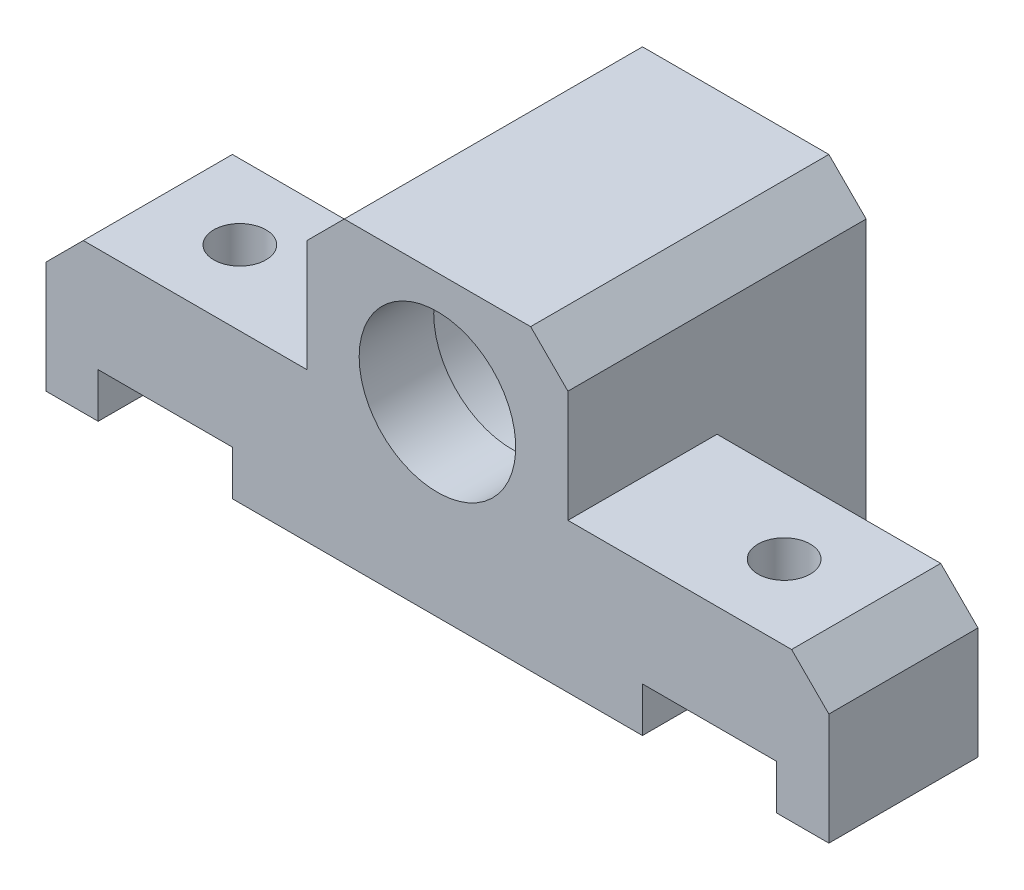
ISO-10303-21;
HEADER;
FILE_DESCRIPTION(('STEP AP214'),'2;1');
FILE_NAME('part.step','',(''),(''),'','','');
FILE_SCHEMA(('AUTOMOTIVE_DESIGN { 1 0 10303 214 1 1 1 1 }'));
ENDSEC;
DATA;
#1=APPLICATION_CONTEXT('core data for automotive mechanical design processes');
#2=APPLICATION_PROTOCOL_DEFINITION('international standard','automotive_design',2000,#1);
#3=PRODUCT_CONTEXT('',#1,'mechanical');
#4=PRODUCT('Part','Part','',(#3));
#5=PRODUCT_RELATED_PRODUCT_CATEGORY('part','',(#4));
#6=PRODUCT_DEFINITION_FORMATION('','',#4);
#7=PRODUCT_DEFINITION_CONTEXT('part definition',#1,'design');
#8=PRODUCT_DEFINITION('design','',#6,#7);
#9=PRODUCT_DEFINITION_SHAPE('','',#8);
#10=(LENGTH_UNIT() NAMED_UNIT(*) SI_UNIT(.MILLI.,.METRE.));
#11=(NAMED_UNIT(*) PLANE_ANGLE_UNIT() SI_UNIT($,.RADIAN.));
#12=(NAMED_UNIT(*) SI_UNIT($,.STERADIAN.) SOLID_ANGLE_UNIT());
#13=UNCERTAINTY_MEASURE_WITH_UNIT(LENGTH_MEASURE(1.E-05),#10,'distance_accuracy_value','');
#14=(GEOMETRIC_REPRESENTATION_CONTEXT(3) GLOBAL_UNCERTAINTY_ASSIGNED_CONTEXT((#13)) GLOBAL_UNIT_ASSIGNED_CONTEXT((#10,
#11,#12)) REPRESENTATION_CONTEXT('',''));
#15=CARTESIAN_POINT('',(0.,0.,0.));
#16=DIRECTION('',(0.,0.,1.));
#17=DIRECTION('',(1.,0.,0.));
#18=AXIS2_PLACEMENT_3D('',#15,#16,#17);
#19=CARTESIAN_POINT('',(0.,0.,40.));
#20=DIRECTION('',(0.,1.,0.));
#21=DIRECTION('',(0.,0.,1.));
#22=AXIS2_PLACEMENT_3D('',#19,#20,#21);
#23=PLANE('',#22);
#24=DIRECTION('',(1.,0.,0.));
#25=VECTOR('',#24,1.);
#26=CARTESIAN_POINT('',(-35.,0.,20.));
#27=LINE('',#26,#25);
#28=CARTESIAN_POINT('',(-35.,0.,20.));
#29=VERTEX_POINT('',#28);
#30=CARTESIAN_POINT('',(-28.,0.,20.));
#31=VERTEX_POINT('',#30);
#32=EDGE_CURVE('E286',#29,#31,#27,.T.);
#33=ORIENTED_EDGE('',*,*,#32,.T.);
#34=DIRECTION('',(0.,0.,-1.));
#35=VECTOR('',#34,1.);
#36=CARTESIAN_POINT('',(-28.,0.,40.));
#37=LINE('',#36,#35);
#38=CARTESIAN_POINT('',(-28.,0.,40.));
#39=VERTEX_POINT('',#38);
#40=EDGE_CURVE('E230',#39,#31,#37,.T.);
#41=ORIENTED_EDGE('',*,*,#40,.F.);
#42=DIRECTION('',(1.,0.,0.));
#43=VECTOR('',#42,1.);
#44=CARTESIAN_POINT('',(0.,0.,40.));
#45=LINE('',#44,#43);
#46=CARTESIAN_POINT('',(-35.,0.,40.));
#47=VERTEX_POINT('',#46);
#48=EDGE_CURVE('E327',#47,#39,#45,.T.);
#49=ORIENTED_EDGE('',*,*,#48,.F.);
#50=DIRECTION('',(0.,0.,1.));
#51=VECTOR('',#50,1.);
#52=CARTESIAN_POINT('',(-35.,0.,20.));
#53=LINE('',#52,#51);
#54=EDGE_CURVE('E313',#29,#47,#53,.T.);
#55=ORIENTED_EDGE('',*,*,#54,.F.);
#56=EDGE_LOOP('',(#33,#41,#49,#55));
#57=FACE_BOUND('',#56,.T.);
#58=ADVANCED_FACE('F44',(#57),#23,.F.);
#59=CARTESIAN_POINT('',(63.,0.,40.));
#60=VERTEX_POINT('',#59);
#61=CARTESIAN_POINT('',(70.,0.,40.));
#62=VERTEX_POINT('',#61);
#63=EDGE_CURVE('E330',#60,#62,#45,.T.);
#64=ORIENTED_EDGE('',*,*,#63,.F.);
#65=DIRECTION('',(0.,0.,-1.));
#66=VECTOR('',#65,1.);
#67=CARTESIAN_POINT('',(63.,0.,40.));
#68=LINE('',#67,#66);
#69=CARTESIAN_POINT('',(63.,0.,20.));
#70=VERTEX_POINT('',#69);
#71=EDGE_CURVE('E250',#60,#70,#68,.T.);
#72=ORIENTED_EDGE('',*,*,#71,.T.);
#73=DIRECTION('',(1.,0.,0.));
#74=VECTOR('',#73,1.);
#75=CARTESIAN_POINT('',(70.,0.,20.));
#76=LINE('',#75,#74);
#77=CARTESIAN_POINT('',(70.,0.,20.));
#78=VERTEX_POINT('',#77);
#79=EDGE_CURVE('E257',#70,#78,#76,.T.);
#80=ORIENTED_EDGE('',*,*,#79,.T.);
#81=DIRECTION('',(0.,0.,1.));
#82=VECTOR('',#81,1.);
#83=CARTESIAN_POINT('',(70.,0.,20.));
#84=LINE('',#83,#82);
#85=EDGE_CURVE('E272',#78,#62,#84,.T.);
#86=ORIENTED_EDGE('',*,*,#85,.T.);
#87=EDGE_LOOP('',(#64,#72,#80,#86));
#88=FACE_BOUND('',#87,.T.);
#89=ADVANCED_FACE('F403',(#88),#23,.F.);
#90=CARTESIAN_POINT('',(35.,0.,40.));
#91=DIRECTION('',(-1.,0.,0.));
#92=DIRECTION('',(0.,0.,1.));
#93=AXIS2_PLACEMENT_3D('',#90,#91,#92);
#94=PLANE('',#93);
#95=DIRECTION('',(0.,0.,1.));
#96=VECTOR('',#95,1.);
#97=CARTESIAN_POINT('',(35.,20.,20.));
#98=LINE('',#97,#96);
#99=CARTESIAN_POINT('',(35.,20.,20.));
#100=VERTEX_POINT('',#99);
#101=CARTESIAN_POINT('',(35.,20.,40.));
#102=VERTEX_POINT('',#101);
#103=EDGE_CURVE('E277',#100,#102,#98,.T.);
#104=ORIENTED_EDGE('',*,*,#103,.F.);
#105=DIRECTION('',(0.,-1.,0.));
#106=VECTOR('',#105,1.);
#107=CARTESIAN_POINT('',(35.,0.,20.));
#108=LINE('',#107,#106);
#109=CARTESIAN_POINT('',(35.,0.,20.));
#110=VERTEX_POINT('',#109);
#111=EDGE_CURVE('E268',#100,#110,#108,.T.);
#112=ORIENTED_EDGE('',*,*,#111,.T.);
#113=DIRECTION('',(0.,0.,-1.));
#114=VECTOR('',#113,1.);
#115=CARTESIAN_POINT('',(35.,0.,40.));
#116=LINE('',#115,#114);
#117=CARTESIAN_POINT('',(35.,0.,0.));
#118=VERTEX_POINT('',#117);
#119=EDGE_CURVE('E52',#110,#118,#116,.T.);
#120=ORIENTED_EDGE('',*,*,#119,.T.);
#121=DIRECTION('',(0.,1.,0.));
#122=VECTOR('',#121,1.);
#123=CARTESIAN_POINT('',(35.,0.,0.));
#124=LINE('',#123,#122);
#125=CARTESIAN_POINT('',(35.,35.,0.));
#126=VERTEX_POINT('',#125);
#127=EDGE_CURVE('E348',#118,#126,#124,.T.);
#128=ORIENTED_EDGE('',*,*,#127,.T.);
#129=DIRECTION('',(0.,0.,-1.));
#130=VECTOR('',#129,1.);
#131=CARTESIAN_POINT('',(35.,35.,40.));
#132=LINE('',#131,#130);
#133=CARTESIAN_POINT('',(35.,35.,40.));
#134=VERTEX_POINT('',#133);
#135=EDGE_CURVE('E363',#134,#126,#132,.T.);
#136=ORIENTED_EDGE('',*,*,#135,.F.);
#137=DIRECTION('',(0.,1.,0.));
#138=VECTOR('',#137,1.);
#139=CARTESIAN_POINT('',(35.,0.,40.));
#140=LINE('',#139,#138);
#141=EDGE_CURVE('E332',#102,#134,#140,.T.);
#142=ORIENTED_EDGE('',*,*,#141,.F.);
#143=EDGE_LOOP('',(#104,#112,#120,#128,#136,#142));
#144=FACE_BOUND('',#143,.T.);
#145=ADVANCED_FACE('F366',(#144),#94,.F.);
#146=CARTESIAN_POINT('',(0.,35.,40.));
#147=DIRECTION('',(1.,0.,0.));
#148=DIRECTION('',(0.,0.,-1.));
#149=AXIS2_PLACEMENT_3D('',#146,#147,#148);
#150=PLANE('',#149);
#151=DIRECTION('',(0.,0.,-1.));
#152=VECTOR('',#151,1.);
#153=CARTESIAN_POINT('',(0.,0.,40.));
#154=LINE('',#153,#152);
#155=CARTESIAN_POINT('',(0.,0.,20.));
#156=VERTEX_POINT('',#155);
#157=CARTESIAN_POINT('',(0.,0.,0.));
#158=VERTEX_POINT('',#157);
#159=EDGE_CURVE('E11',#156,#158,#154,.T.);
#160=ORIENTED_EDGE('',*,*,#159,.F.);
#161=DIRECTION('',(0.,1.,0.));
#162=VECTOR('',#161,1.);
#163=CARTESIAN_POINT('',(0.,0.,20.));
#164=LINE('',#163,#162);
#165=CARTESIAN_POINT('',(0.,20.,20.));
#166=VERTEX_POINT('',#165);
#167=EDGE_CURVE('E291',#156,#166,#164,.T.);
#168=ORIENTED_EDGE('',*,*,#167,.T.);
#169=DIRECTION('',(0.,0.,1.));
#170=VECTOR('',#169,1.);
#171=CARTESIAN_POINT('',(0.,20.,20.));
#172=LINE('',#171,#170);
#173=CARTESIAN_POINT('',(0.,20.,40.));
#174=VERTEX_POINT('',#173);
#175=EDGE_CURVE('E304',#166,#174,#172,.T.);
#176=ORIENTED_EDGE('',*,*,#175,.T.);
#177=DIRECTION('',(0.,-1.,0.));
#178=VECTOR('',#177,1.);
#179=CARTESIAN_POINT('',(0.,35.,40.));
#180=LINE('',#179,#178);
#181=CARTESIAN_POINT('',(0.,35.,40.));
#182=VERTEX_POINT('',#181);
#183=EDGE_CURVE('E323',#182,#174,#180,.T.);
#184=ORIENTED_EDGE('',*,*,#183,.F.);
#185=DIRECTION('',(0.,0.,-1.));
#186=VECTOR('',#185,1.);
#187=CARTESIAN_POINT('',(0.,35.,40.));
#188=LINE('',#187,#186);
#189=CARTESIAN_POINT('',(0.,35.,0.));
#190=VERTEX_POINT('',#189);
#191=EDGE_CURVE('E338',#182,#190,#188,.T.);
#192=ORIENTED_EDGE('',*,*,#191,.T.);
#193=DIRECTION('',(0.,-1.,0.));
#194=VECTOR('',#193,1.);
#195=CARTESIAN_POINT('',(0.,35.,0.));
#196=LINE('',#195,#194);
#197=EDGE_CURVE('E320',#190,#158,#196,.T.);
#198=ORIENTED_EDGE('',*,*,#197,.T.);
#199=EDGE_LOOP('',(#160,#168,#176,#184,#192,#198));
#200=FACE_BOUND('',#199,.T.);
#201=ADVANCED_FACE('F50',(#200),#150,.F.);
#202=CARTESIAN_POINT('',(-9.99999999999999,0.,40.));
#203=VERTEX_POINT('',#202);
#204=CARTESIAN_POINT('',(45.,0.,40.));
#205=VERTEX_POINT('',#204);
#206=EDGE_CURVE('E335',#203,#205,#45,.T.);
#207=ORIENTED_EDGE('',*,*,#206,.F.);
#208=DIRECTION('',(0.,0.,-1.));
#209=VECTOR('',#208,1.);
#210=CARTESIAN_POINT('',(-9.99999999999999,0.,40.));
#211=LINE('',#210,#209);
#212=CARTESIAN_POINT('',(-9.99999999999999,0.,20.));
#213=VERTEX_POINT('',#212);
#214=EDGE_CURVE('E202',#203,#213,#211,.T.);
#215=ORIENTED_EDGE('',*,*,#214,.T.);
#216=EDGE_CURVE('E295',#213,#156,#27,.T.);
#217=ORIENTED_EDGE('',*,*,#216,.T.);
#218=ORIENTED_EDGE('',*,*,#159,.T.);
#219=DIRECTION('',(1.,0.,0.));
#220=VECTOR('',#219,1.);
#221=CARTESIAN_POINT('',(0.,0.,0.));
#222=LINE('',#221,#220);
#223=EDGE_CURVE('E345',#158,#118,#222,.T.);
#224=ORIENTED_EDGE('',*,*,#223,.T.);
#225=ORIENTED_EDGE('',*,*,#119,.F.);
#226=CARTESIAN_POINT('',(45.,0.,20.));
#227=VERTEX_POINT('',#226);
#228=EDGE_CURVE('E259',#110,#227,#76,.T.);
#229=ORIENTED_EDGE('',*,*,#228,.T.);
#230=DIRECTION('',(0.,0.,-1.));
#231=VECTOR('',#230,1.);
#232=CARTESIAN_POINT('',(45.,0.,40.));
#233=LINE('',#232,#231);
#234=EDGE_CURVE('E66',#205,#227,#233,.T.);
#235=ORIENTED_EDGE('',*,*,#234,.F.);
#236=EDGE_LOOP('',(#207,#215,#217,#218,#224,#225,#229,#235));
#237=FACE_BOUND('',#236,.T.);
#238=ADVANCED_FACE('F375',(#237),#23,.F.);
#239=CARTESIAN_POINT('',(35.,35.,40.));
#240=DIRECTION('',(-0.707106781186548,-0.707106781186548,0.));
#241=DIRECTION('',(0.707106781186548,-0.707106781186548,0.));
#242=AXIS2_PLACEMENT_3D('',#239,#240,#241);
#243=PLANE('',#242);
#244=DIRECTION('',(-0.707106781186547,0.707106781186547,0.));
#245=VECTOR('',#244,1.);
#246=CARTESIAN_POINT('',(35.,35.,0.));
#247=LINE('',#246,#245);
#248=CARTESIAN_POINT('',(30.,40.,0.));
#249=VERTEX_POINT('',#248);
#250=EDGE_CURVE('E346',#126,#249,#247,.T.);
#251=ORIENTED_EDGE('',*,*,#250,.T.);
#252=DIRECTION('',(0.,0.,-1.));
#253=VECTOR('',#252,1.);
#254=CARTESIAN_POINT('',(30.,40.,40.));
#255=LINE('',#254,#253);
#256=CARTESIAN_POINT('',(30.,40.,40.));
#257=VERTEX_POINT('',#256);
#258=EDGE_CURVE('E356',#257,#249,#255,.T.);
#259=ORIENTED_EDGE('',*,*,#258,.F.);
#260=DIRECTION('',(-0.707106781186547,0.707106781186547,0.));
#261=VECTOR('',#260,1.);
#262=CARTESIAN_POINT('',(35.,35.,40.));
#263=LINE('',#262,#261);
#264=EDGE_CURVE('E334',#134,#257,#263,.T.);
#265=ORIENTED_EDGE('',*,*,#264,.F.);
#266=ORIENTED_EDGE('',*,*,#135,.T.);
#267=EDGE_LOOP('',(#251,#259,#265,#266));
#268=FACE_BOUND('',#267,.T.);
#269=ADVANCED_FACE('F385',(#268),#243,.F.);
#270=CARTESIAN_POINT('',(30.,40.,40.));
#271=DIRECTION('',(0.,-1.,0.));
#272=DIRECTION('',(0.,0.,-1.));
#273=AXIS2_PLACEMENT_3D('',#270,#271,#272);
#274=PLANE('',#273);
#275=DIRECTION('',(-1.,0.,0.));
#276=VECTOR('',#275,1.);
#277=CARTESIAN_POINT('',(30.,40.,0.));
#278=LINE('',#277,#276);
#279=CARTESIAN_POINT('',(5.,40.,0.));
#280=VERTEX_POINT('',#279);
#281=EDGE_CURVE('E349',#249,#280,#278,.T.);
#282=ORIENTED_EDGE('',*,*,#281,.T.);
#283=DIRECTION('',(0.,0.,-1.));
#284=VECTOR('',#283,1.);
#285=CARTESIAN_POINT('',(5.,40.,40.));
#286=LINE('',#285,#284);
#287=CARTESIAN_POINT('',(5.,40.,40.));
#288=VERTEX_POINT('',#287);
#289=EDGE_CURVE('E351',#288,#280,#286,.T.);
#290=ORIENTED_EDGE('',*,*,#289,.F.);
#291=DIRECTION('',(-1.,0.,0.));
#292=VECTOR('',#291,1.);
#293=CARTESIAN_POINT('',(30.,40.,40.));
#294=LINE('',#293,#292);
#295=EDGE_CURVE('E337',#257,#288,#294,.T.);
#296=ORIENTED_EDGE('',*,*,#295,.F.);
#297=ORIENTED_EDGE('',*,*,#258,.T.);
#298=EDGE_LOOP('',(#282,#290,#296,#297));
#299=FACE_BOUND('',#298,.T.);
#300=ADVANCED_FACE('F389',(#299),#274,.F.);
#301=CARTESIAN_POINT('',(5.,40.,40.));
#302=DIRECTION('',(0.707106781186547,-0.707106781186548,0.));
#303=DIRECTION('',(0.707106781186548,0.707106781186547,0.));
#304=AXIS2_PLACEMENT_3D('',#301,#302,#303);
#305=PLANE('',#304);
#306=DIRECTION('',(-0.707106781186548,-0.707106781186547,0.));
#307=VECTOR('',#306,1.);
#308=CARTESIAN_POINT('',(5.,40.,0.));
#309=LINE('',#308,#307);
#310=EDGE_CURVE('E326',#280,#190,#309,.T.);
#311=ORIENTED_EDGE('',*,*,#310,.T.);
#312=ORIENTED_EDGE('',*,*,#191,.F.);
#313=DIRECTION('',(-0.707106781186548,-0.707106781186547,0.));
#314=VECTOR('',#313,1.);
#315=CARTESIAN_POINT('',(5.,40.,40.));
#316=LINE('',#315,#314);
#317=EDGE_CURVE('E336',#288,#182,#316,.T.);
#318=ORIENTED_EDGE('',*,*,#317,.F.);
#319=ORIENTED_EDGE('',*,*,#289,.T.);
#320=EDGE_LOOP('',(#311,#312,#318,#319));
#321=FACE_BOUND('',#320,.T.);
#322=ADVANCED_FACE('F451',(#321),#305,.F.);
#323=CARTESIAN_POINT('',(0.,0.,40.));
#324=DIRECTION('',(0.,0.,1.));
#325=DIRECTION('',(1.,0.,0.));
#326=AXIS2_PLACEMENT_3D('',#323,#324,#325);
#327=PLANE('',#326);
#328=CARTESIAN_POINT('',(17.5,25.,40.));
#329=DIRECTION('',(0.,0.,-1.));
#330=DIRECTION('',(-1.,0.,0.));
#331=AXIS2_PLACEMENT_3D('',#328,#329,#330);
#332=CIRCLE('',#331,10.5);
#333=CARTESIAN_POINT('',(7.,25.,40.));
#334=VERTEX_POINT('',#333);
#335=EDGE_CURVE('E876',#334,#334,#332,.T.);
#336=ORIENTED_EDGE('',*,*,#335,.T.);
#337=EDGE_LOOP('',(#336));
#338=FACE_BOUND('',#337,.T.);
#339=DIRECTION('',(0.,1.,0.));
#340=VECTOR('',#339,1.);
#341=CARTESIAN_POINT('',(-28.,0.,40.));
#342=LINE('',#341,#340);
#343=CARTESIAN_POINT('',(-28.,6.,40.));
#344=VERTEX_POINT('',#343);
#345=EDGE_CURVE('E205',#39,#344,#342,.T.);
#346=ORIENTED_EDGE('',*,*,#345,.T.);
#347=DIRECTION('',(1.,0.,0.));
#348=VECTOR('',#347,1.);
#349=CARTESIAN_POINT('',(0.,6.,40.));
#350=LINE('',#349,#348);
#351=CARTESIAN_POINT('',(-9.99999999999999,6.,40.));
#352=VERTEX_POINT('',#351);
#353=EDGE_CURVE('E200',#344,#352,#350,.T.);
#354=ORIENTED_EDGE('',*,*,#353,.T.);
#355=DIRECTION('',(0.,-1.,0.));
#356=VECTOR('',#355,1.);
#357=CARTESIAN_POINT('',(-9.99999999999999,0.,40.));
#358=LINE('',#357,#356);
#359=EDGE_CURVE('E201',#352,#203,#358,.T.);
#360=ORIENTED_EDGE('',*,*,#359,.T.);
#361=ORIENTED_EDGE('',*,*,#206,.T.);
#362=DIRECTION('',(0.,1.,0.));
#363=VECTOR('',#362,1.);
#364=CARTESIAN_POINT('',(45.,6.,40.));
#365=LINE('',#364,#363);
#366=CARTESIAN_POINT('',(45.,6.,40.));
#367=VERTEX_POINT('',#366);
#368=EDGE_CURVE('E235',#205,#367,#365,.T.);
#369=ORIENTED_EDGE('',*,*,#368,.T.);
#370=DIRECTION('',(1.,0.,0.));
#371=VECTOR('',#370,1.);
#372=CARTESIAN_POINT('',(63.,6.,40.));
#373=LINE('',#372,#371);
#374=CARTESIAN_POINT('',(63.,6.,40.));
#375=VERTEX_POINT('',#374);
#376=EDGE_CURVE('E232',#367,#375,#373,.T.);
#377=ORIENTED_EDGE('',*,*,#376,.T.);
#378=DIRECTION('',(0.,-1.,0.));
#379=VECTOR('',#378,1.);
#380=CARTESIAN_POINT('',(63.,0.,40.));
#381=LINE('',#380,#379);
#382=EDGE_CURVE('E237',#375,#60,#381,.T.);
#383=ORIENTED_EDGE('',*,*,#382,.T.);
#384=ORIENTED_EDGE('',*,*,#63,.T.);
#385=DIRECTION('',(0.,1.,0.));
#386=VECTOR('',#385,1.);
#387=CARTESIAN_POINT('',(70.,15.,40.));
#388=LINE('',#387,#386);
#389=CARTESIAN_POINT('',(70.,15.,40.));
#390=VERTEX_POINT('',#389);
#391=EDGE_CURVE('E249',#62,#390,#388,.T.);
#392=ORIENTED_EDGE('',*,*,#391,.T.);
#393=DIRECTION('',(-0.707106781186547,0.707106781186548,0.));
#394=VECTOR('',#393,1.);
#395=CARTESIAN_POINT('',(70.,15.,40.));
#396=LINE('',#395,#394);
#397=CARTESIAN_POINT('',(64.9999999999999,20.0000000000001,40.));
#398=VERTEX_POINT('',#397);
#399=EDGE_CURVE('E274',#390,#398,#396,.T.);
#400=ORIENTED_EDGE('',*,*,#399,.T.);
#401=DIRECTION('',(-1.,0.,0.));
#402=VECTOR('',#401,1.);
#403=CARTESIAN_POINT('',(35.,20.,40.));
#404=LINE('',#403,#402);
#405=EDGE_CURVE('E276',#398,#102,#404,.T.);
#406=ORIENTED_EDGE('',*,*,#405,.T.);
#407=ORIENTED_EDGE('',*,*,#141,.T.);
#408=ORIENTED_EDGE('',*,*,#264,.T.);
#409=ORIENTED_EDGE('',*,*,#295,.T.);
#410=ORIENTED_EDGE('',*,*,#317,.T.);
#411=ORIENTED_EDGE('',*,*,#183,.T.);
#412=DIRECTION('',(-1.,0.,0.));
#413=VECTOR('',#412,1.);
#414=CARTESIAN_POINT('',(-28.,20.,40.));
#415=LINE('',#414,#413);
#416=CARTESIAN_POINT('',(-30.,20.,40.));
#417=VERTEX_POINT('',#416);
#418=EDGE_CURVE('E285',#174,#417,#415,.T.);
#419=ORIENTED_EDGE('',*,*,#418,.T.);
#420=DIRECTION('',(-0.707106781186546,-0.707106781186549,0.));
#421=VECTOR('',#420,1.);
#422=CARTESIAN_POINT('',(-35.,15.,40.));
#423=LINE('',#422,#421);
#424=CARTESIAN_POINT('',(-35.,15.,40.));
#425=VERTEX_POINT('',#424);
#426=EDGE_CURVE('E308',#417,#425,#423,.T.);
#427=ORIENTED_EDGE('',*,*,#426,.T.);
#428=DIRECTION('',(0.,-1.,0.));
#429=VECTOR('',#428,1.);
#430=CARTESIAN_POINT('',(-35.,15.,40.));
#431=LINE('',#430,#429);
#432=EDGE_CURVE('E311',#425,#47,#431,.T.);
#433=ORIENTED_EDGE('',*,*,#432,.T.);
#434=ORIENTED_EDGE('',*,*,#48,.T.);
#435=EDGE_LOOP('',(#346,#354,#360,#361,#369,#377,#383,#384,#392,#400,#406,#407,#408,#409,#410,
#411,#419,#427,#433,#434));
#436=FACE_BOUND('',#435,.T.);
#437=ADVANCED_FACE('F214',(#338,#436),#327,.T.);
#438=CARTESIAN_POINT('',(0.,0.,0.));
#439=DIRECTION('',(0.,0.,1.));
#440=DIRECTION('',(1.,0.,0.));
#441=AXIS2_PLACEMENT_3D('',#438,#439,#440);
#442=PLANE('',#441);
#443=CARTESIAN_POINT('',(17.5,25.,0.));
#444=DIRECTION('',(0.,0.,-1.));
#445=DIRECTION('',(-1.,0.,0.));
#446=AXIS2_PLACEMENT_3D('',#443,#444,#445);
#447=CIRCLE('',#446,14.5);
#448=CARTESIAN_POINT('',(3.,25.,0.));
#449=VERTEX_POINT('',#448);
#450=EDGE_CURVE('E871',#449,#449,#447,.T.);
#451=ORIENTED_EDGE('',*,*,#450,.F.);
#452=EDGE_LOOP('',(#451));
#453=FACE_BOUND('',#452,.T.);
#454=ORIENTED_EDGE('',*,*,#197,.F.);
#455=ORIENTED_EDGE('',*,*,#310,.F.);
#456=ORIENTED_EDGE('',*,*,#281,.F.);
#457=ORIENTED_EDGE('',*,*,#250,.F.);
#458=ORIENTED_EDGE('',*,*,#127,.F.);
#459=ORIENTED_EDGE('',*,*,#223,.F.);
#460=EDGE_LOOP('',(#454,#455,#456,#457,#458,#459));
#461=FACE_BOUND('',#460,.T.);
#462=ADVANCED_FACE('F380',(#453,#461),#442,.F.);
#463=CARTESIAN_POINT('',(-35.,15.,20.));
#464=DIRECTION('',(-1.,0.,0.));
#465=DIRECTION('',(0.,0.,1.));
#466=AXIS2_PLACEMENT_3D('',#463,#464,#465);
#467=PLANE('',#466);
#468=ORIENTED_EDGE('',*,*,#432,.F.);
#469=DIRECTION('',(0.,0.,1.));
#470=VECTOR('',#469,1.);
#471=CARTESIAN_POINT('',(-35.,15.,20.));
#472=LINE('',#471,#470);
#473=CARTESIAN_POINT('',(-35.,15.,20.));
#474=VERTEX_POINT('',#473);
#475=EDGE_CURVE('E319',#474,#425,#472,.T.);
#476=ORIENTED_EDGE('',*,*,#475,.F.);
#477=DIRECTION('',(0.,-1.,0.));
#478=VECTOR('',#477,1.);
#479=CARTESIAN_POINT('',(-35.,15.,20.));
#480=LINE('',#479,#478);
#481=EDGE_CURVE('E305',#474,#29,#480,.T.);
#482=ORIENTED_EDGE('',*,*,#481,.T.);
#483=ORIENTED_EDGE('',*,*,#54,.T.);
#484=EDGE_LOOP('',(#468,#476,#482,#483));
#485=FACE_BOUND('',#484,.T.);
#486=ADVANCED_FACE('F464',(#485),#467,.T.);
#487=CARTESIAN_POINT('',(-35.,15.,20.));
#488=DIRECTION('',(-0.707106781186549,0.707106781186546,0.));
#489=DIRECTION('',(-0.707106781186546,-0.707106781186549,0.));
#490=AXIS2_PLACEMENT_3D('',#487,#488,#489);
#491=PLANE('',#490);
#492=ORIENTED_EDGE('',*,*,#426,.F.);
#493=DIRECTION('',(0.,0.,1.));
#494=VECTOR('',#493,1.);
#495=CARTESIAN_POINT('',(-30.,20.,20.));
#496=LINE('',#495,#494);
#497=CARTESIAN_POINT('',(-30.,20.,20.));
#498=VERTEX_POINT('',#497);
#499=EDGE_CURVE('E318',#498,#417,#496,.T.);
#500=ORIENTED_EDGE('',*,*,#499,.F.);
#501=DIRECTION('',(-0.707106781186546,-0.707106781186549,0.));
#502=VECTOR('',#501,1.);
#503=CARTESIAN_POINT('',(-35.,15.,20.));
#504=LINE('',#503,#502);
#505=EDGE_CURVE('E299',#498,#474,#504,.T.);
#506=ORIENTED_EDGE('',*,*,#505,.T.);
#507=ORIENTED_EDGE('',*,*,#475,.T.);
#508=EDGE_LOOP('',(#492,#500,#506,#507));
#509=FACE_BOUND('',#508,.T.);
#510=ADVANCED_FACE('F462',(#509),#491,.T.);
#511=CARTESIAN_POINT('',(-28.,20.,20.));
#512=DIRECTION('',(0.,1.,0.));
#513=DIRECTION('',(0.,0.,1.));
#514=AXIS2_PLACEMENT_3D('',#511,#512,#513);
#515=PLANE('',#514);
#516=CARTESIAN_POINT('',(-19.,20.,30.));
#517=DIRECTION('',(0.,1.,0.));
#518=DIRECTION('',(0.,0.,1.));
#519=AXIS2_PLACEMENT_3D('',#516,#517,#518);
#520=CIRCLE('',#519,3.5);
#521=CARTESIAN_POINT('',(-19.,20.,33.5));
#522=VERTEX_POINT('',#521);
#523=EDGE_CURVE('E860',#522,#522,#520,.T.);
#524=ORIENTED_EDGE('',*,*,#523,.F.);
#525=EDGE_LOOP('',(#524));
#526=FACE_BOUND('',#525,.T.);
#527=ORIENTED_EDGE('',*,*,#418,.F.);
#528=ORIENTED_EDGE('',*,*,#175,.F.);
#529=DIRECTION('',(-1.,0.,0.));
#530=VECTOR('',#529,1.);
#531=CARTESIAN_POINT('',(0.,20.,20.));
#532=LINE('',#531,#530);
#533=EDGE_CURVE('E300',#166,#498,#532,.T.);
#534=ORIENTED_EDGE('',*,*,#533,.T.);
#535=ORIENTED_EDGE('',*,*,#499,.T.);
#536=EDGE_LOOP('',(#527,#528,#534,#535));
#537=FACE_BOUND('',#536,.T.);
#538=ADVANCED_FACE('F458',(#526,#537),#515,.T.);
#539=CARTESIAN_POINT('',(0.,0.,20.));
#540=DIRECTION('',(0.,0.,1.));
#541=DIRECTION('',(1.,0.,0.));
#542=AXIS2_PLACEMENT_3D('',#539,#540,#541);
#543=PLANE('',#542);
#544=DIRECTION('',(1.,0.,0.));
#545=VECTOR('',#544,1.);
#546=CARTESIAN_POINT('',(0.,6.,20.));
#547=LINE('',#546,#545);
#548=CARTESIAN_POINT('',(-28.,6.,20.));
#549=VERTEX_POINT('',#548);
#550=CARTESIAN_POINT('',(-9.99999999999999,6.,20.));
#551=VERTEX_POINT('',#550);
#552=EDGE_CURVE('E58',#549,#551,#547,.T.);
#553=ORIENTED_EDGE('',*,*,#552,.F.);
#554=DIRECTION('',(0.,1.,0.));
#555=VECTOR('',#554,1.);
#556=CARTESIAN_POINT('',(-28.,0.,20.));
#557=LINE('',#556,#555);
#558=EDGE_CURVE('E215',#31,#549,#557,.T.);
#559=ORIENTED_EDGE('',*,*,#558,.F.);
#560=ORIENTED_EDGE('',*,*,#32,.F.);
#561=ORIENTED_EDGE('',*,*,#481,.F.);
#562=ORIENTED_EDGE('',*,*,#505,.F.);
#563=ORIENTED_EDGE('',*,*,#533,.F.);
#564=ORIENTED_EDGE('',*,*,#167,.F.);
#565=ORIENTED_EDGE('',*,*,#216,.F.);
#566=DIRECTION('',(0.,-1.,0.));
#567=VECTOR('',#566,1.);
#568=CARTESIAN_POINT('',(-9.99999999999999,0.,20.));
#569=LINE('',#568,#567);
#570=EDGE_CURVE('E218',#551,#213,#569,.T.);
#571=ORIENTED_EDGE('',*,*,#570,.F.);
#572=EDGE_LOOP('',(#553,#559,#560,#561,#562,#563,#564,#565,#571));
#573=FACE_BOUND('',#572,.T.);
#574=ADVANCED_FACE('F468',(#573),#543,.F.);
#575=CARTESIAN_POINT('',(35.,20.,20.));
#576=DIRECTION('',(0.,1.,0.));
#577=DIRECTION('',(0.,0.,1.));
#578=AXIS2_PLACEMENT_3D('',#575,#576,#577);
#579=PLANE('',#578);
#580=CARTESIAN_POINT('',(54.,20.,30.));
#581=DIRECTION('',(0.,1.,0.));
#582=DIRECTION('',(0.,0.,1.));
#583=AXIS2_PLACEMENT_3D('',#580,#581,#582);
#584=CIRCLE('',#583,3.50000000000001);
#585=CARTESIAN_POINT('',(54.,20.,33.5));
#586=VERTEX_POINT('',#585);
#587=EDGE_CURVE('E217',#586,#586,#584,.T.);
#588=ORIENTED_EDGE('',*,*,#587,.F.);
#589=EDGE_LOOP('',(#588));
#590=FACE_BOUND('',#589,.T.);
#591=ORIENTED_EDGE('',*,*,#405,.F.);
#592=DIRECTION('',(0.,0.,1.));
#593=VECTOR('',#592,1.);
#594=CARTESIAN_POINT('',(64.9999999999999,20.0000000000001,20.));
#595=LINE('',#594,#593);
#596=CARTESIAN_POINT('',(64.9999999999999,20.0000000000001,20.));
#597=VERTEX_POINT('',#596);
#598=EDGE_CURVE('E281',#597,#398,#595,.T.);
#599=ORIENTED_EDGE('',*,*,#598,.F.);
#600=DIRECTION('',(-1.,0.,0.));
#601=VECTOR('',#600,1.);
#602=CARTESIAN_POINT('',(63.,20.,20.));
#603=LINE('',#602,#601);
#604=EDGE_CURVE('E267',#597,#100,#603,.T.);
#605=ORIENTED_EDGE('',*,*,#604,.T.);
#606=ORIENTED_EDGE('',*,*,#103,.T.);
#607=EDGE_LOOP('',(#591,#599,#605,#606));
#608=FACE_BOUND('',#607,.T.);
#609=ADVANCED_FACE('F395',(#590,#608),#579,.T.);
#610=CARTESIAN_POINT('',(70.,15.,20.));
#611=DIRECTION('',(0.707106781186548,0.707106781186547,0.));
#612=DIRECTION('',(-0.707106781186547,0.707106781186548,0.));
#613=AXIS2_PLACEMENT_3D('',#610,#611,#612);
#614=PLANE('',#613);
#615=ORIENTED_EDGE('',*,*,#399,.F.);
#616=DIRECTION('',(0.,0.,1.));
#617=VECTOR('',#616,1.);
#618=CARTESIAN_POINT('',(70.,15.,20.));
#619=LINE('',#618,#617);
#620=CARTESIAN_POINT('',(70.,15.,20.));
#621=VERTEX_POINT('',#620);
#622=EDGE_CURVE('E287',#621,#390,#619,.T.);
#623=ORIENTED_EDGE('',*,*,#622,.F.);
#624=DIRECTION('',(-0.707106781186547,0.707106781186548,0.));
#625=VECTOR('',#624,1.);
#626=CARTESIAN_POINT('',(70.,15.,20.));
#627=LINE('',#626,#625);
#628=EDGE_CURVE('E261',#621,#597,#627,.T.);
#629=ORIENTED_EDGE('',*,*,#628,.T.);
#630=ORIENTED_EDGE('',*,*,#598,.T.);
#631=EDGE_LOOP('',(#615,#623,#629,#630));
#632=FACE_BOUND('',#631,.T.);
#633=ADVANCED_FACE('F415',(#632),#614,.T.);
#634=CARTESIAN_POINT('',(70.,15.,20.));
#635=DIRECTION('',(1.,0.,0.));
#636=DIRECTION('',(0.,0.,-1.));
#637=AXIS2_PLACEMENT_3D('',#634,#635,#636);
#638=PLANE('',#637);
#639=ORIENTED_EDGE('',*,*,#391,.F.);
#640=ORIENTED_EDGE('',*,*,#85,.F.);
#641=DIRECTION('',(0.,1.,0.));
#642=VECTOR('',#641,1.);
#643=CARTESIAN_POINT('',(70.,15.,20.));
#644=LINE('',#643,#642);
#645=EDGE_CURVE('E258',#78,#621,#644,.T.);
#646=ORIENTED_EDGE('',*,*,#645,.T.);
#647=ORIENTED_EDGE('',*,*,#622,.T.);
#648=EDGE_LOOP('',(#639,#640,#646,#647));
#649=FACE_BOUND('',#648,.T.);
#650=ADVANCED_FACE('F408',(#649),#638,.T.);
#651=CARTESIAN_POINT('',(0.,0.,20.));
#652=DIRECTION('',(0.,0.,-1.));
#653=DIRECTION('',(-1.,0.,0.));
#654=AXIS2_PLACEMENT_3D('',#651,#652,#653);
#655=PLANE('',#654);
#656=DIRECTION('',(0.,-1.,0.));
#657=VECTOR('',#656,1.);
#658=CARTESIAN_POINT('',(63.,0.,20.));
#659=LINE('',#658,#657);
#660=CARTESIAN_POINT('',(63.,6.,20.));
#661=VERTEX_POINT('',#660);
#662=EDGE_CURVE('E236',#661,#70,#659,.T.);
#663=ORIENTED_EDGE('',*,*,#662,.F.);
#664=DIRECTION('',(1.,0.,0.));
#665=VECTOR('',#664,1.);
#666=CARTESIAN_POINT('',(63.,6.,20.));
#667=LINE('',#666,#665);
#668=CARTESIAN_POINT('',(45.,6.,20.));
#669=VERTEX_POINT('',#668);
#670=EDGE_CURVE('E243',#669,#661,#667,.T.);
#671=ORIENTED_EDGE('',*,*,#670,.F.);
#672=DIRECTION('',(0.,1.,0.));
#673=VECTOR('',#672,1.);
#674=CARTESIAN_POINT('',(45.,6.,20.));
#675=LINE('',#674,#673);
#676=EDGE_CURVE('E226',#227,#669,#675,.T.);
#677=ORIENTED_EDGE('',*,*,#676,.F.);
#678=ORIENTED_EDGE('',*,*,#228,.F.);
#679=ORIENTED_EDGE('',*,*,#111,.F.);
#680=ORIENTED_EDGE('',*,*,#604,.F.);
#681=ORIENTED_EDGE('',*,*,#628,.F.);
#682=ORIENTED_EDGE('',*,*,#645,.F.);
#683=ORIENTED_EDGE('',*,*,#79,.F.);
#684=EDGE_LOOP('',(#663,#671,#677,#678,#679,#680,#681,#682,#683));
#685=FACE_BOUND('',#684,.T.);
#686=ADVANCED_FACE('F400',(#685),#655,.T.);
#687=CARTESIAN_POINT('',(63.,0.,40.));
#688=DIRECTION('',(1.,0.,0.));
#689=DIRECTION('',(0.,0.,-1.));
#690=AXIS2_PLACEMENT_3D('',#687,#688,#689);
#691=PLANE('',#690);
#692=ORIENTED_EDGE('',*,*,#662,.T.);
#693=ORIENTED_EDGE('',*,*,#71,.F.);
#694=ORIENTED_EDGE('',*,*,#382,.F.);
#695=DIRECTION('',(0.,0.,-1.));
#696=VECTOR('',#695,1.);
#697=CARTESIAN_POINT('',(63.,6.,40.));
#698=LINE('',#697,#696);
#699=EDGE_CURVE('E252',#375,#661,#698,.T.);
#700=ORIENTED_EDGE('',*,*,#699,.T.);
#701=EDGE_LOOP('',(#692,#693,#694,#700));
#702=FACE_BOUND('',#701,.T.);
#703=ADVANCED_FACE('F412',(#702),#691,.F.);
#704=CARTESIAN_POINT('',(63.,6.,40.));
#705=DIRECTION('',(0.,1.,0.));
#706=DIRECTION('',(0.,0.,1.));
#707=AXIS2_PLACEMENT_3D('',#704,#705,#706);
#708=PLANE('',#707);
#709=CARTESIAN_POINT('',(54.,6.,30.));
#710=DIRECTION('',(0.,1.,0.));
#711=DIRECTION('',(0.,0.,1.));
#712=AXIS2_PLACEMENT_3D('',#709,#710,#711);
#713=CIRCLE('',#712,2.5);
#714=CARTESIAN_POINT('',(54.,6.,32.5));
#715=VERTEX_POINT('',#714);
#716=EDGE_CURVE('E847',#715,#715,#713,.T.);
#717=ORIENTED_EDGE('',*,*,#716,.T.);
#718=EDGE_LOOP('',(#717));
#719=FACE_BOUND('',#718,.T.);
#720=ORIENTED_EDGE('',*,*,#670,.T.);
#721=ORIENTED_EDGE('',*,*,#699,.F.);
#722=ORIENTED_EDGE('',*,*,#376,.F.);
#723=DIRECTION('',(0.,0.,-1.));
#724=VECTOR('',#723,1.);
#725=CARTESIAN_POINT('',(45.,6.,40.));
#726=LINE('',#725,#724);
#727=EDGE_CURVE('E254',#367,#669,#726,.T.);
#728=ORIENTED_EDGE('',*,*,#727,.T.);
#729=EDGE_LOOP('',(#720,#721,#722,#728));
#730=FACE_BOUND('',#729,.T.);
#731=ADVANCED_FACE('F420',(#719,#730),#708,.F.);
#732=CARTESIAN_POINT('',(45.,6.,40.));
#733=DIRECTION('',(-1.,0.,0.));
#734=DIRECTION('',(0.,0.,1.));
#735=AXIS2_PLACEMENT_3D('',#732,#733,#734);
#736=PLANE('',#735);
#737=ORIENTED_EDGE('',*,*,#676,.T.);
#738=ORIENTED_EDGE('',*,*,#727,.F.);
#739=ORIENTED_EDGE('',*,*,#368,.F.);
#740=ORIENTED_EDGE('',*,*,#234,.T.);
#741=EDGE_LOOP('',(#737,#738,#739,#740));
#742=FACE_BOUND('',#741,.T.);
#743=ADVANCED_FACE('F418',(#742),#736,.F.);
#744=CARTESIAN_POINT('',(0.,6.,40.));
#745=DIRECTION('',(0.,1.,0.));
#746=DIRECTION('',(0.,0.,1.));
#747=AXIS2_PLACEMENT_3D('',#744,#745,#746);
#748=PLANE('',#747);
#749=CARTESIAN_POINT('',(-19.,6.,30.));
#750=DIRECTION('',(0.,1.,0.));
#751=DIRECTION('',(0.,0.,1.));
#752=AXIS2_PLACEMENT_3D('',#749,#750,#751);
#753=CIRCLE('',#752,2.5);
#754=CARTESIAN_POINT('',(-19.,6.,32.5));
#755=VERTEX_POINT('',#754);
#756=EDGE_CURVE('E870',#755,#755,#753,.T.);
#757=ORIENTED_EDGE('',*,*,#756,.T.);
#758=EDGE_LOOP('',(#757));
#759=FACE_BOUND('',#758,.T.);
#760=ORIENTED_EDGE('',*,*,#552,.T.);
#761=DIRECTION('',(0.,0.,-1.));
#762=VECTOR('',#761,1.);
#763=CARTESIAN_POINT('',(-9.99999999999999,6.,40.));
#764=LINE('',#763,#762);
#765=EDGE_CURVE('E195',#352,#551,#764,.T.);
#766=ORIENTED_EDGE('',*,*,#765,.F.);
#767=ORIENTED_EDGE('',*,*,#353,.F.);
#768=DIRECTION('',(0.,0.,-1.));
#769=VECTOR('',#768,1.);
#770=CARTESIAN_POINT('',(-28.,6.,40.));
#771=LINE('',#770,#769);
#772=EDGE_CURVE('E228',#344,#549,#771,.T.);
#773=ORIENTED_EDGE('',*,*,#772,.T.);
#774=EDGE_LOOP('',(#760,#766,#767,#773));
#775=FACE_BOUND('',#774,.T.);
#776=ADVANCED_FACE('F192',(#759,#775),#748,.F.);
#777=CARTESIAN_POINT('',(-28.,0.,40.));
#778=DIRECTION('',(-1.,0.,0.));
#779=DIRECTION('',(0.,0.,1.));
#780=AXIS2_PLACEMENT_3D('',#777,#778,#779);
#781=PLANE('',#780);
#782=ORIENTED_EDGE('',*,*,#558,.T.);
#783=ORIENTED_EDGE('',*,*,#772,.F.);
#784=ORIENTED_EDGE('',*,*,#345,.F.);
#785=ORIENTED_EDGE('',*,*,#40,.T.);
#786=EDGE_LOOP('',(#782,#783,#784,#785));
#787=FACE_BOUND('',#786,.T.);
#788=ADVANCED_FACE('F428',(#787),#781,.F.);
#789=CARTESIAN_POINT('',(-9.99999999999999,0.,40.));
#790=DIRECTION('',(1.,0.,0.));
#791=DIRECTION('',(0.,0.,-1.));
#792=AXIS2_PLACEMENT_3D('',#789,#790,#791);
#793=PLANE('',#792);
#794=ORIENTED_EDGE('',*,*,#570,.T.);
#795=ORIENTED_EDGE('',*,*,#214,.F.);
#796=ORIENTED_EDGE('',*,*,#359,.F.);
#797=ORIENTED_EDGE('',*,*,#765,.T.);
#798=EDGE_LOOP('',(#794,#795,#796,#797));
#799=FACE_BOUND('',#798,.T.);
#800=ADVANCED_FACE('F207',(#799),#793,.F.);
#801=CARTESIAN_POINT('',(54.,13.,30.));
#802=DIRECTION('',(0.,1.,0.));
#803=DIRECTION('',(0.,0.,1.));
#804=AXIS2_PLACEMENT_3D('',#801,#802,#803);
#805=CYLINDRICAL_SURFACE('',#804,3.50000000000001);
#806=CARTESIAN_POINT('',(54.,13.,30.));
#807=DIRECTION('',(0.,1.,0.));
#808=DIRECTION('',(0.,0.,1.));
#809=AXIS2_PLACEMENT_3D('',#806,#807,#808);
#810=CIRCLE('',#809,3.50000000000001);
#811=CARTESIAN_POINT('',(54.,13.,33.5));
#812=VERTEX_POINT('',#811);
#813=EDGE_CURVE('E224',#812,#812,#810,.T.);
#814=ORIENTED_EDGE('',*,*,#813,.F.);
#815=EDGE_LOOP('',(#814));
#816=FACE_BOUND('',#815,.T.);
#817=ORIENTED_EDGE('',*,*,#587,.T.);
#818=EDGE_LOOP('',(#817));
#819=FACE_BOUND('',#818,.T.);
#820=ADVANCED_FACE('F518',(#816,#819),#805,.F.);
#821=CARTESIAN_POINT('',(54.,13.,30.));
#822=DIRECTION('',(0.,1.,0.));
#823=DIRECTION('',(0.,0.,1.));
#824=AXIS2_PLACEMENT_3D('',#821,#822,#823);
#825=PLANE('',#824);
#826=CARTESIAN_POINT('',(54.,13.,30.));
#827=DIRECTION('',(0.,1.,0.));
#828=DIRECTION('',(0.,0.,1.));
#829=AXIS2_PLACEMENT_3D('',#826,#827,#828);
#830=CIRCLE('',#829,2.5);
#831=CARTESIAN_POINT('',(54.,13.,32.5));
#832=VERTEX_POINT('',#831);
#833=EDGE_CURVE('E855',#832,#832,#830,.T.);
#834=ORIENTED_EDGE('',*,*,#833,.F.);
#835=EDGE_LOOP('',(#834));
#836=FACE_BOUND('',#835,.T.);
#837=ORIENTED_EDGE('',*,*,#813,.T.);
#838=EDGE_LOOP('',(#837));
#839=FACE_BOUND('',#838,.T.);
#840=ADVANCED_FACE('F525',(#836,#839),#825,.T.);
#841=CARTESIAN_POINT('',(54.,6.,30.));
#842=DIRECTION('',(0.,1.,0.));
#843=DIRECTION('',(0.,0.,1.));
#844=AXIS2_PLACEMENT_3D('',#841,#842,#843);
#845=CYLINDRICAL_SURFACE('',#844,2.5);
#846=ORIENTED_EDGE('',*,*,#716,.F.);
#847=EDGE_LOOP('',(#846));
#848=FACE_BOUND('',#847,.T.);
#849=ORIENTED_EDGE('',*,*,#833,.T.);
#850=EDGE_LOOP('',(#849));
#851=FACE_BOUND('',#850,.T.);
#852=ADVANCED_FACE('F526',(#848,#851),#845,.F.);
#853=CARTESIAN_POINT('',(-19.,13.,30.));
#854=DIRECTION('',(0.,1.,0.));
#855=DIRECTION('',(0.,0.,1.));
#856=AXIS2_PLACEMENT_3D('',#853,#854,#855);
#857=CYLINDRICAL_SURFACE('',#856,3.5);
#858=CARTESIAN_POINT('',(-19.,13.,30.));
#859=DIRECTION('',(0.,1.,0.));
#860=DIRECTION('',(0.,0.,1.));
#861=AXIS2_PLACEMENT_3D('',#858,#859,#860);
#862=CIRCLE('',#861,3.5);
#863=CARTESIAN_POINT('',(-19.,13.,33.5));
#864=VERTEX_POINT('',#863);
#865=EDGE_CURVE('E853',#864,#864,#862,.T.);
#866=ORIENTED_EDGE('',*,*,#865,.F.);
#867=EDGE_LOOP('',(#866));
#868=FACE_BOUND('',#867,.T.);
#869=ORIENTED_EDGE('',*,*,#523,.T.);
#870=EDGE_LOOP('',(#869));
#871=FACE_BOUND('',#870,.T.);
#872=ADVANCED_FACE('F539',(#868,#871),#857,.F.);
#873=CARTESIAN_POINT('',(-19.,13.,30.));
#874=DIRECTION('',(0.,1.,0.));
#875=DIRECTION('',(0.,0.,1.));
#876=AXIS2_PLACEMENT_3D('',#873,#874,#875);
#877=PLANE('',#876);
#878=CARTESIAN_POINT('',(-19.,13.,30.));
#879=DIRECTION('',(0.,1.,0.));
#880=DIRECTION('',(0.,0.,1.));
#881=AXIS2_PLACEMENT_3D('',#878,#879,#880);
#882=CIRCLE('',#881,2.5);
#883=CARTESIAN_POINT('',(-19.,13.,32.5));
#884=VERTEX_POINT('',#883);
#885=EDGE_CURVE('E867',#884,#884,#882,.T.);
#886=ORIENTED_EDGE('',*,*,#885,.F.);
#887=EDGE_LOOP('',(#886));
#888=FACE_BOUND('',#887,.T.);
#889=ORIENTED_EDGE('',*,*,#865,.T.);
#890=EDGE_LOOP('',(#889));
#891=FACE_BOUND('',#890,.T.);
#892=ADVANCED_FACE('F538',(#888,#891),#877,.T.);
#893=CARTESIAN_POINT('',(-19.,6.,30.));
#894=DIRECTION('',(0.,1.,0.));
#895=DIRECTION('',(0.,0.,1.));
#896=AXIS2_PLACEMENT_3D('',#893,#894,#895);
#897=CYLINDRICAL_SURFACE('',#896,2.5);
#898=ORIENTED_EDGE('',*,*,#756,.F.);
#899=EDGE_LOOP('',(#898));
#900=FACE_BOUND('',#899,.T.);
#901=ORIENTED_EDGE('',*,*,#885,.T.);
#902=EDGE_LOOP('',(#901));
#903=FACE_BOUND('',#902,.T.);
#904=ADVANCED_FACE('F550',(#900,#903),#897,.F.);
#905=CARTESIAN_POINT('',(17.5,25.,30.));
#906=DIRECTION('',(0.,0.,-1.));
#907=DIRECTION('',(-1.,0.,0.));
#908=AXIS2_PLACEMENT_3D('',#905,#906,#907);
#909=CYLINDRICAL_SURFACE('',#908,14.5);
#910=CARTESIAN_POINT('',(17.5,25.,30.));
#911=DIRECTION('',(0.,0.,-1.));
#912=DIRECTION('',(-1.,0.,0.));
#913=AXIS2_PLACEMENT_3D('',#910,#911,#912);
#914=CIRCLE('',#913,14.5);
#915=CARTESIAN_POINT('',(3.,25.,30.));
#916=VERTEX_POINT('',#915);
#917=EDGE_CURVE('E875',#916,#916,#914,.T.);
#918=ORIENTED_EDGE('',*,*,#917,.F.);
#919=EDGE_LOOP('',(#918));
#920=FACE_BOUND('',#919,.T.);
#921=ORIENTED_EDGE('',*,*,#450,.T.);
#922=EDGE_LOOP('',(#921));
#923=FACE_BOUND('',#922,.T.);
#924=ADVANCED_FACE('F551',(#920,#923),#909,.F.);
#925=CARTESIAN_POINT('',(17.5,25.,30.));
#926=DIRECTION('',(0.,0.,-1.));
#927=DIRECTION('',(-1.,0.,0.));
#928=AXIS2_PLACEMENT_3D('',#925,#926,#927);
#929=PLANE('',#928);
#930=CARTESIAN_POINT('',(17.5,25.,30.));
#931=DIRECTION('',(0.,0.,-1.));
#932=DIRECTION('',(-1.,0.,0.));
#933=AXIS2_PLACEMENT_3D('',#930,#931,#932);
#934=CIRCLE('',#933,10.5);
#935=CARTESIAN_POINT('',(7.,25.,30.));
#936=VERTEX_POINT('',#935);
#937=EDGE_CURVE('E883',#936,#936,#934,.T.);
#938=ORIENTED_EDGE('',*,*,#937,.F.);
#939=EDGE_LOOP('',(#938));
#940=FACE_BOUND('',#939,.T.);
#941=ORIENTED_EDGE('',*,*,#917,.T.);
#942=EDGE_LOOP('',(#941));
#943=FACE_BOUND('',#942,.T.);
#944=ADVANCED_FACE('F558',(#940,#943),#929,.T.);
#945=CARTESIAN_POINT('',(17.5,25.,40.));
#946=DIRECTION('',(0.,0.,-1.));
#947=DIRECTION('',(-1.,0.,0.));
#948=AXIS2_PLACEMENT_3D('',#945,#946,#947);
#949=CYLINDRICAL_SURFACE('',#948,10.5);
#950=ORIENTED_EDGE('',*,*,#335,.F.);
#951=EDGE_LOOP('',(#950));
#952=FACE_BOUND('',#951,.T.);
#953=ORIENTED_EDGE('',*,*,#937,.T.);
#954=EDGE_LOOP('',(#953));
#955=FACE_BOUND('',#954,.T.);
#956=ADVANCED_FACE('F563',(#952,#955),#949,.F.);
#957=CLOSED_SHELL('',(#58,#89,#145,#201,#238,#269,#300,#322,#437,#462,#486,#510,#538,#574,#609,
#633,#650,#686,#703,#731,#743,#776,#788,#800,#820,#840,#852,#872,#892,#904,#924,#944,#956));
#958=MANIFOLD_SOLID_BREP('B2',#957);
#959=ADVANCED_BREP_SHAPE_REPRESENTATION('',(#18,#958),#14);
#960=SHAPE_DEFINITION_REPRESENTATION(#9,#959);
ENDSEC;
END-ISO-10303-21;
